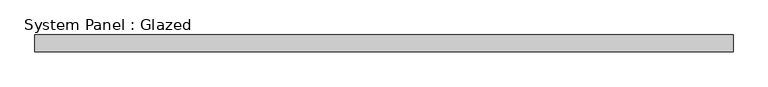
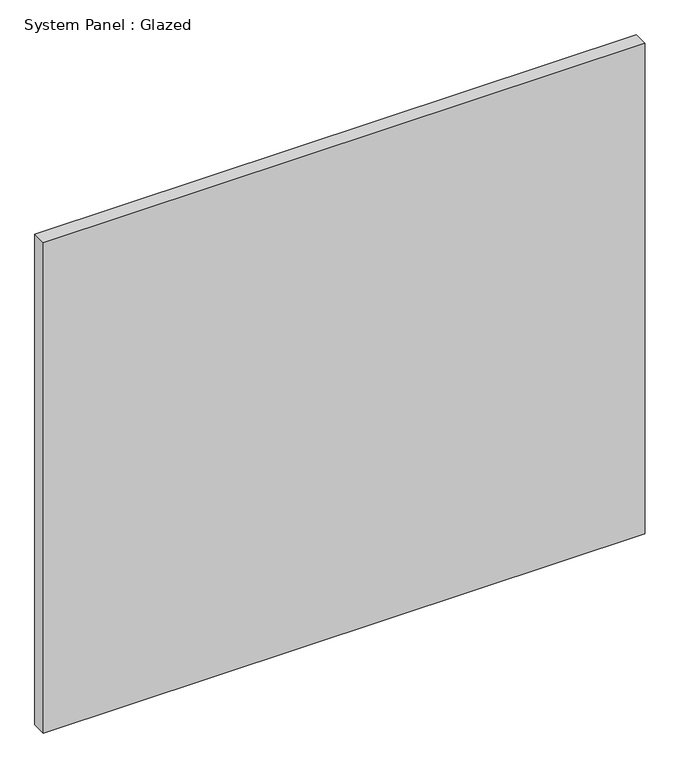
"""IFC4 building model written with IfcOpenShell, lengths in millimetres: plate geometry, System Panel : Glazed."""

from ifc_helpers import new_model, si_unit, origin, origin_with_axes, place, context, project, spatial, polyline, outline, extrude, source, transform, mapped, element, save


def system_panel_glazed_8b2f71d4(model_context):
    return source(origin(), model_context, "Body", "SweptSolid", [
        extrude(outline(polyline([(520.9254305, 19.05), (-520.9254305, 19.05), (-520.9254305, 44.45), (520.9254305, 44.45), (520.9254305, 19.05)])), origin_with_axes(), (0.0, 0.0, 1.0), 897.5064813),
    ])


if __name__ == "__main__":
    model = new_model("IFC4")
    model_context = context("Model", 3, world=origin())
    ifc_project = project(units=[si_unit("LENGTHUNIT", "METRE", prefix="MILLI")], contexts=[model_context])
    site = spatial("IfcSite", under=ifc_project)
    building = spatial("IfcBuilding", under=site)
    placement = place(None, origin())
    system_panel_glazed_shape = system_panel_glazed_8b2f71d4(model_context)
    element("IfcPlate", 1, ObjectType="System Panel : Glazed", at=placement, inside=building, context=model_context, shape_type="MappedRepresentation", body=[
        mapped(system_panel_glazed_shape, transform((0.0, 0.0, 0.0), x_axis=(1.0, 0.0, 0.0), y_axis=(0.0, 1.0, 0.0), z_axis=(0.0, 0.0, 1.0))),
    ])
    save(model, "model.ifc")

# Revit data of these elements
# Type "System Panel : Glazed"
#   Construction Type Id = "GSP4R"
#   Analytic Construction = "1/8 in Pilkington single glazing"
#   Visual Light Transmittance = 0.9
#   Solar Heat Gain Coefficient = 0.86
#   Heat Transfer Coefficient (U) = 1.18115 BTU/(h·ft²·°F)
#   Define Thermal Properties by = 1
# Element 1 (IfcPlate, "System Panel : Glazed")
#   Materials on its faces: "Glass"
# Materials
#   "Glass": class "Glass", colour RGB 0 128 192, transparency 0.75, Description = "Soda Lime Glass", Cost = 0
